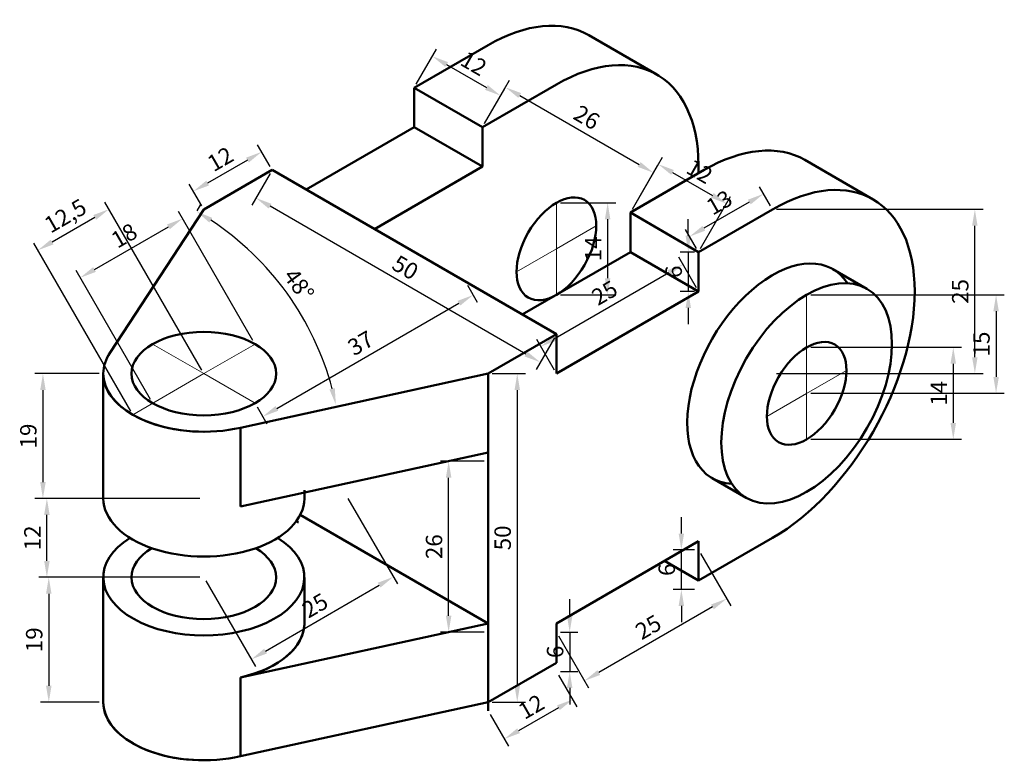
# Model space of a CAD drawing. Units: millimetres. Extents: x 225 to 375, y 60 to 173.
import ezdxf

# ---------------------------------------------------------------- set-up
doc = ezdxf.new("R2010")
doc.units = ezdxf.units.MM
doc.linetypes.add('CENTER', pattern=[50.8, 31.75, -6.35, 6.35, -6.35])
for name, color, linetype, lineweight in [('M-CNTR', 1, 'CENTER', 18), ('M-DIMS', 2, 'Continuous', 25), ('M-OUTL', 7, 'Continuous', 50)]:
    doc.layers.add(name, color=color, linetype=linetype, lineweight=lineweight)
doc.styles.get("Standard").update_dxf_attribs({"font": 'arial.ttf'})
doc.dimstyles.new('ISO-25', dxfattribs={"dimtxt": 2.5, "dimasz": 2.5, "dimexe": 1.25, "dimexo": 0.625, "dimtad": 1, "dimtxsty": 'Standard', "dimcen": 2.5, "dimadec": 0, "dimazin": 0, "dimtfac": 1, "dimtmove": 0, "dimatfit": 3, "dimfxl": 1, "dimarcsym": 0})

# ---------------------------------------------------------------- blocks, each defined once
blk = doc.blocks.new('*D1')
at = {"layer": 'Defpoints', "color": 0, "transparency": 16777216}
for p in [(252.15, 143.3), (269.41, 126), (238.15, 119.06), (296.76, 119.06), (253.46, 110.22)]:
    blk.add_point(p, dxfattribs=at)
at = {"layer": 'M-DIMS', "color": 0, "lineweight": -2, "transparency": 16777216}
blk.add_line((252.46, 143.84), (253.02, 144.8), dxfattribs=at)
blk.add_arc((230.32, 105.49), 44.14, 14.7826, 56.7544, dxfattribs=at)
at = {"layer": 'M-DIMS', "color": 0, "transparency": 16777216}
for points in [[(254.3, 142.05), (254.74, 142.76), (252.39, 143.72)], [(273.41, 116.85), (272.59, 116.66), (273.57, 114.32)]]:
    blk.add_solid(points, dxfattribs=at)
at = {"layer": 'M-DIMS', "color": 0, "transparency": 16777216, "insert": (267.68, 132.4), "char_height": 2.5, "attachment_point": 5, "rotation": 305.7685}
blk.add_mtext('48°', dxfattribs=at)
blk = doc.blocks.new('*D2')
at = {"layer": 'Defpoints', "color": 0, "transparency": 16777216}
for p in [(263.85, 150.06), (261.39, 145.79), (307.15, 125.06)]:
    blk.add_point(p, dxfattribs=at)
at = {"layer": 'M-DIMS', "color": 0, "lineweight": -2, "transparency": 16777216}
for p, q in [((263.54, 149.51), (260.76, 144.7)), ((302.52, 122.04), (263.55, 144.54)), ((306.84, 124.51), (304.06, 119.7))]:
    blk.add_line(p, q, dxfattribs=at)
at = {"layer": 'M-DIMS', "color": 0, "transparency": 16777216}
for points in [[(263.76, 144.9), (263.35, 144.17), (261.39, 145.79)], [(302.73, 122.4), (302.32, 121.67), (304.69, 120.79)]]:
    blk.add_solid(points, dxfattribs=at)
at = {"layer": 'M-DIMS', "color": 0, "transparency": 16777216, "insert": (283.99, 134.93), "char_height": 2.5, "attachment_point": 5, "rotation": 330}
blk.add_mtext('50', dxfattribs=at)
blk = doc.blocks.new('*D3')
at = {"layer": 'Defpoints', "color": 0, "transparency": 16777216}
for p in [(296.76, 119.06), (296.76, 69.06), (301.19, 69.06)]:
    blk.add_point(p, dxfattribs=at)
at = {"layer": 'M-DIMS', "color": 0, "lineweight": -2, "transparency": 16777216}
for p, q in [((297.39, 119.06), (302.44, 119.06)), ((301.19, 116.56), (301.19, 71.56)), ((297.39, 69.06), (302.44, 69.06))]:
    blk.add_line(p, q, dxfattribs=at)
at = {"layer": 'M-DIMS', "color": 0, "transparency": 16777216}
for points in [[(300.78, 116.56), (301.61, 116.56), (301.19, 119.06)], [(300.78, 71.56), (301.61, 71.56), (301.19, 69.06)]]:
    blk.add_solid(points, dxfattribs=at)
at = {"layer": 'M-DIMS', "color": 0, "transparency": 16777216, "insert": (299.29, 94.06), "char_height": 2.5, "attachment_point": 5, "rotation": 90}
blk.add_mtext('50', dxfattribs=at)
blk = doc.blocks.new('*D4')
at = {"layer": 'Defpoints', "color": 0, "transparency": 16777216}
for p in [(307.15, 79.72), (307.15, 73.72), (309.18, 73.72)]:
    blk.add_point(p, dxfattribs=at)
at = {"layer": 'M-DIMS', "color": 0, "lineweight": -2, "transparency": 16777216}
for p, q in [((309.18, 82.22), (309.18, 84.72)), ((307.78, 79.72), (310.43, 79.72)), ((309.18, 79.72), (309.18, 73.72)), ((307.78, 73.72), (310.43, 73.72)), ((309.18, 71.22), (309.18, 68.72))]:
    blk.add_line(p, q, dxfattribs=at)
at = {"layer": 'M-DIMS', "color": 0, "transparency": 16777216}
for points in [[(308.76, 82.22), (309.6, 82.22), (309.18, 79.72)], [(308.76, 71.22), (309.6, 71.22), (309.18, 73.72)]]:
    blk.add_solid(points, dxfattribs=at)
at = {"layer": 'M-DIMS', "color": 0, "transparency": 16777216, "insert": (307.28, 76.72), "char_height": 2.5, "attachment_point": 5, "rotation": 90}
blk.add_mtext('6', dxfattribs=at)
blk = doc.blocks.new('*D5')
at = {"layer": 'Defpoints', "color": 0, "transparency": 16777216}
for p in [(328.81, 92.22), (307.15, 79.72), (311.43, 72.31)]:
    blk.add_point(p, dxfattribs=at)
at = {"layer": 'M-DIMS', "color": 0, "lineweight": -2, "transparency": 16777216}
for p, q in [((329.12, 91.68), (333.71, 83.73)), ((330.92, 83.56), (313.6, 73.56)), ((307.47, 79.18), (312.06, 71.23))]:
    blk.add_line(p, q, dxfattribs=at)
at = {"layer": 'M-DIMS', "color": 0, "transparency": 16777216}
for points in [[(330.71, 83.92), (331.13, 83.2), (333.08, 84.81)], [(313.39, 73.92), (313.81, 73.2), (311.43, 72.31)]]:
    blk.add_solid(points, dxfattribs=at)
at = {"layer": 'M-DIMS', "color": 0, "transparency": 16777216, "insert": (321.31, 80.21), "char_height": 2.5, "attachment_point": 5, "rotation": 30}
blk.add_mtext('25', dxfattribs=at)
blk = doc.blocks.new('*D6')
at = {"layer": 'Defpoints', "color": 0, "transparency": 16777216}
for p in [(326.18, 92.22), (328.81, 92.22), (328.81, 86.22)]:
    blk.add_point(p, dxfattribs=at)
at = {"layer": 'M-DIMS', "color": 0, "lineweight": -2, "transparency": 16777216}
for p, q in [((326.18, 94.72), (326.18, 97.22)), ((328.18, 92.22), (324.93, 92.22)), ((326.18, 86.22), (326.18, 92.22)), ((328.18, 86.22), (324.93, 86.22)), ((326.18, 83.72), (326.18, 81.22))]:
    blk.add_line(p, q, dxfattribs=at)
at = {"layer": 'M-DIMS', "color": 0, "transparency": 16777216}
for points in [[(325.77, 94.72), (326.6, 94.72), (326.18, 92.22)], [(325.77, 83.72), (326.6, 83.72), (326.18, 86.22)]]:
    blk.add_solid(points, dxfattribs=at)
at = {"layer": 'M-DIMS', "color": 0, "transparency": 16777216, "insert": (324.28, 89.22), "char_height": 2.5, "attachment_point": 5, "rotation": 90}
blk.add_mtext('6', dxfattribs=at)
blk = doc.blocks.new('*D7')
at = {"layer": 'Defpoints', "color": 0, "transparency": 16777216}
for p in [(345.26, 123.06), (345.26, 109.06), (367.59, 109.06)]:
    blk.add_point(p, dxfattribs=at)
at = {"layer": 'M-DIMS', "color": 0, "lineweight": -2, "transparency": 16777216}
for p, q in [((345.88, 123.06), (368.84, 123.06)), ((367.59, 120.56), (367.59, 111.56)), ((345.88, 109.06), (368.84, 109.06))]:
    blk.add_line(p, q, dxfattribs=at)
at = {"layer": 'M-DIMS', "color": 0, "transparency": 16777216}
for points in [[(367.17, 120.56), (368.01, 120.56), (367.59, 123.06)], [(367.17, 111.56), (368.01, 111.56), (367.59, 109.06)]]:
    blk.add_solid(points, dxfattribs=at)
at = {"layer": 'M-DIMS', "color": 0, "transparency": 16777216, "insert": (365.71, 116.06), "char_height": 2.5, "attachment_point": 5, "rotation": 90}
blk.add_mtext('14', dxfattribs=at)
blk = doc.blocks.new('*D8')
at = {"layer": 'Defpoints', "color": 0, "transparency": 16777216}
for p in [(345.26, 131.06), (345.26, 116.06), (374.11, 116.06)]:
    blk.add_point(p, dxfattribs=at)
at = {"layer": 'M-DIMS', "color": 0, "lineweight": -2, "transparency": 16777216}
for p, q in [((345.88, 131.06), (375.36, 131.06)), ((374.11, 128.56), (374.11, 118.56)), ((345.88, 116.06), (375.36, 116.06))]:
    blk.add_line(p, q, dxfattribs=at)
at = {"layer": 'M-DIMS', "color": 0, "transparency": 16777216}
for points in [[(373.7, 128.56), (374.53, 128.56), (374.11, 131.06)], [(373.7, 118.56), (374.53, 118.56), (374.11, 116.06)]]:
    blk.add_solid(points, dxfattribs=at)
at = {"layer": 'M-DIMS', "color": 0, "transparency": 16777216, "insert": (372.21, 123.56), "char_height": 2.5, "attachment_point": 5, "rotation": 90}
blk.add_mtext('15', dxfattribs=at)
blk = doc.blocks.new('*D9')
at = {"layer": 'Defpoints', "color": 0, "transparency": 16777216}
for p in [(340.06, 144.06), (327.44, 139.92), (328.81, 137.56)]:
    blk.add_point(p, dxfattribs=at)
at = {"layer": 'M-DIMS', "color": 0, "lineweight": -2, "transparency": 16777216}
for p, q in [((339.75, 144.6), (338.07, 147.5)), ((336.53, 145.17), (329.61, 141.17)), ((328.49, 138.1), (326.82, 141))]:
    blk.add_line(p, q, dxfattribs=at)
at = {"layer": 'M-DIMS', "color": 0, "transparency": 16777216}
for points in [[(336.33, 145.53), (336.74, 144.81), (338.7, 146.42)], [(329.4, 141.53), (329.81, 140.81), (327.44, 139.92)]]:
    blk.add_solid(points, dxfattribs=at)
at = {"layer": 'M-DIMS', "color": 0, "transparency": 16777216, "insert": (332.12, 144.82), "char_height": 2.5, "attachment_point": 5, "rotation": 30}
blk.add_mtext('13', dxfattribs=at)
blk = doc.blocks.new('*D10')
at = {"layer": 'Defpoints', "color": 0, "transparency": 16777216}
for p in [(328.81, 137.56), (327.24, 131.56), (328.81, 131.56)]:
    blk.add_point(p, dxfattribs=at)
at = {"layer": 'M-DIMS', "color": 0, "lineweight": -2, "transparency": 16777216}
for p, q in [((327.24, 140.06), (327.24, 142.56)), ((328.18, 137.56), (325.99, 137.56)), ((327.24, 137.56), (327.24, 131.56)), ((328.18, 131.56), (325.99, 131.56)), ((327.24, 129.06), (327.24, 126.56))]:
    blk.add_line(p, q, dxfattribs=at)
at = {"layer": 'M-DIMS', "color": 0, "transparency": 16777216}
for points in [[(326.82, 140.06), (327.65, 140.06), (327.24, 137.56)], [(326.82, 129.06), (327.65, 129.06), (327.24, 131.56)]]:
    blk.add_solid(points, dxfattribs=at)
at = {"layer": 'M-DIMS', "color": 0, "transparency": 16777216, "insert": (325.34, 134.56), "char_height": 2.5, "attachment_point": 5, "rotation": 90}
blk.add_mtext('6', dxfattribs=at)
blk = doc.blocks.new('*D11')
at = {"layer": 'Defpoints', "color": 0, "transparency": 16777216}
for p in [(326.43, 135.68), (328.81, 131.56), (307.15, 119.06)]:
    blk.add_point(p, dxfattribs=at)
at = {"layer": 'M-DIMS', "color": 0, "lineweight": -2, "transparency": 16777216}
for p, q in [((328.49, 132.1), (325.8, 136.76)), ((306.94, 124.43), (324.26, 134.43)), ((306.84, 119.6), (304.15, 124.26))]:
    blk.add_line(p, q, dxfattribs=at)
at = {"layer": 'M-DIMS', "color": 0, "transparency": 16777216}
for points in [[(324.05, 134.79), (324.47, 134.07), (326.43, 135.68)], [(306.73, 124.79), (307.15, 124.07), (304.78, 123.18)]]:
    blk.add_solid(points, dxfattribs=at)
at = {"layer": 'M-DIMS', "color": 0, "transparency": 16777216, "insert": (314.65, 131.07), "char_height": 2.5, "attachment_point": 5, "rotation": 30}
blk.add_mtext('25', dxfattribs=at)
blk = doc.blocks.new('*D12')
at = {"layer": 'Defpoints', "color": 0, "transparency": 16777216}
for p in [(295.9, 156.56), (321.92, 149.63), (318.41, 143.56)]:
    blk.add_point(p, dxfattribs=at)
at = {"layer": 'M-DIMS', "color": 0, "lineweight": -2, "transparency": 16777216}
for p, q in [((296.21, 157.1), (300.03, 163.72)), ((301.57, 161.38), (319.76, 150.88)), ((318.73, 144.1), (322.55, 150.72))]:
    blk.add_line(p, q, dxfattribs=at)
at = {"layer": 'M-DIMS', "color": 0, "transparency": 16777216}
for points in [[(301.78, 161.75), (301.36, 161.02), (299.41, 162.63)], [(319.97, 151.25), (319.55, 150.52), (321.92, 149.63)]]:
    blk.add_solid(points, dxfattribs=at)
at = {"layer": 'M-DIMS', "color": 0, "transparency": 16777216, "insert": (311.62, 157.78), "char_height": 2.5, "attachment_point": 5, "rotation": 330}
blk.add_mtext('26', dxfattribs=at)
blk = doc.blocks.new('*D13')
at = {"layer": 'Defpoints', "color": 0, "transparency": 16777216}
for p in [(333.06, 144.93), (318.41, 143.56), (328.81, 137.56)]:
    blk.add_point(p, dxfattribs=at)
at = {"layer": 'M-DIMS', "color": 0, "lineweight": -2, "transparency": 16777216}
for p, q in [((318.73, 144.1), (323.3, 152.01)), ((324.84, 149.68), (330.9, 146.18)), ((329.12, 138.1), (333.69, 146.01))]:
    blk.add_line(p, q, dxfattribs=at)
at = {"layer": 'M-DIMS', "color": 0, "transparency": 16777216}
for points in [[(325.04, 150.04), (324.63, 149.32), (322.67, 150.93)], [(331.11, 146.54), (330.69, 145.82), (333.06, 144.93)]]:
    blk.add_solid(points, dxfattribs=at)
at = {"layer": 'M-DIMS', "color": 0, "transparency": 16777216, "insert": (328.81, 149.56), "char_height": 2.5, "attachment_point": 5, "rotation": 330}
blk.add_mtext('12', dxfattribs=at)
blk = doc.blocks.new('*D14')
at = {"layer": 'Defpoints', "color": 0, "transparency": 16777216}
for p in [(285.5, 162.56), (298.66, 161.35), (295.9, 156.56)]:
    blk.add_point(p, dxfattribs=at)
at = {"layer": 'M-DIMS', "color": 0, "lineweight": -2, "transparency": 16777216}
for p, q in [((285.82, 163.1), (288.9, 168.43)), ((290.44, 166.1), (296.5, 162.6)), ((296.21, 157.1), (299.29, 162.43))]:
    blk.add_line(p, q, dxfattribs=at)
at = {"layer": 'M-DIMS', "color": 0, "transparency": 16777216}
for points in [[(290.64, 166.46), (290.23, 165.74), (288.27, 167.35)], [(296.71, 162.96), (296.29, 162.24), (298.66, 161.35)]]:
    blk.add_solid(points, dxfattribs=at)
at = {"layer": 'M-DIMS', "color": 0, "transparency": 16777216, "insert": (294.41, 165.98), "char_height": 2.5, "attachment_point": 5, "rotation": 330}
blk.add_mtext('12', dxfattribs=at)
blk = doc.blocks.new('*D15')
at = {"layer": 'Defpoints', "color": 0, "transparency": 16777216}
for p in [(307.15, 145.06), (307.15, 131.06), (314.96, 131.06)]:
    blk.add_point(p, dxfattribs=at)
at = {"layer": 'M-DIMS', "color": 0, "lineweight": -2, "transparency": 16777216}
for p, q in [((307.78, 145.06), (316.21, 145.06)), ((314.96, 142.56), (314.96, 133.56)), ((307.78, 131.06), (316.21, 131.06))]:
    blk.add_line(p, q, dxfattribs=at)
at = {"layer": 'M-DIMS', "color": 0, "transparency": 16777216}
for points in [[(314.54, 142.56), (315.37, 142.56), (314.96, 145.06)], [(314.54, 133.56), (315.37, 133.56), (314.96, 131.06)]]:
    blk.add_solid(points, dxfattribs=at)
at = {"layer": 'M-DIMS', "color": 0, "transparency": 16777216, "insert": (313.08, 138.06), "char_height": 2.5, "attachment_point": 5, "rotation": 90}
blk.add_mtext('14', dxfattribs=at)
blk = doc.blocks.new('*D16')
at = {"layer": 'Defpoints', "color": 0, "transparency": 16777216}
for p in [(238.15, 119.06), (228.96, 100.06), (238.15, 100.06)]:
    blk.add_point(p, dxfattribs=at)
at = {"layer": 'M-DIMS', "color": 0, "lineweight": -2, "transparency": 16777216}
for p, q in [((237.53, 119.06), (227.71, 119.06)), ((228.96, 116.56), (228.96, 102.56)), ((237.53, 100.06), (227.71, 100.06))]:
    blk.add_line(p, q, dxfattribs=at)
at = {"layer": 'M-DIMS', "color": 0, "transparency": 16777216}
for points in [[(228.54, 116.56), (229.38, 116.56), (228.96, 119.06)], [(228.54, 102.56), (229.38, 102.56), (228.96, 100.06)]]:
    blk.add_solid(points, dxfattribs=at)
at = {"layer": 'M-DIMS', "color": 0, "transparency": 16777216, "insert": (227.06, 109.56), "char_height": 2.5, "attachment_point": 5, "rotation": 90}
blk.add_mtext('19', dxfattribs=at)
blk = doc.blocks.new('*D17')
at = {"layer": 'Defpoints', "color": 0, "transparency": 16777216}
for p in [(238.15, 88.06), (229.85, 69.06), (238.15, 69.06)]:
    blk.add_point(p, dxfattribs=at)
at = {"layer": 'M-DIMS', "color": 0, "lineweight": -2, "transparency": 16777216}
for p, q in [((237.53, 88.06), (228.6, 88.06)), ((229.85, 85.56), (229.85, 71.56)), ((237.53, 69.06), (228.6, 69.06))]:
    blk.add_line(p, q, dxfattribs=at)
at = {"layer": 'M-DIMS', "color": 0, "transparency": 16777216}
for points in [[(229.43, 85.56), (230.27, 85.56), (229.85, 88.06)], [(229.43, 71.56), (230.27, 71.56), (229.85, 69.06)]]:
    blk.add_solid(points, dxfattribs=at)
at = {"layer": 'M-DIMS', "color": 0, "transparency": 16777216, "insert": (227.95, 78.56), "char_height": 2.5, "attachment_point": 5, "rotation": 90}
blk.add_mtext('19', dxfattribs=at)
blk = doc.blocks.new('*D18')
at = {"layer": 'Defpoints', "color": 0, "transparency": 16777216}
for p in [(290.74, 105.72), (296.76, 105.72), (296.76, 79.72)]:
    blk.add_point(p, dxfattribs=at)
at = {"layer": 'M-DIMS', "color": 0, "lineweight": -2, "transparency": 16777216}
for p, q in [((296.14, 105.72), (289.49, 105.72)), ((290.74, 82.22), (290.74, 103.22)), ((296.14, 79.72), (289.49, 79.72))]:
    blk.add_line(p, q, dxfattribs=at)
at = {"layer": 'M-DIMS', "color": 0, "transparency": 16777216}
for points in [[(290.32, 103.22), (291.16, 103.22), (290.74, 105.72)], [(290.32, 82.22), (291.16, 82.22), (290.74, 79.72)]]:
    blk.add_solid(points, dxfattribs=at)
at = {"layer": 'M-DIMS', "color": 0, "transparency": 16777216, "insert": (288.84, 92.72), "char_height": 2.5, "attachment_point": 5, "rotation": 90}
blk.add_mtext('26', dxfattribs=at)
blk = doc.blocks.new('*D19')
at = {"layer": 'Defpoints', "color": 0, "transparency": 16777216}
for p in [(275.08, 100.6), (253.46, 88.06), (282.32, 88.13)]:
    blk.add_point(p, dxfattribs=at)
at = {"layer": 'M-DIMS', "color": 0, "lineweight": -2, "transparency": 16777216}
for p, q in [((275.4, 100.06), (282.95, 87.05)), ((253.77, 87.51), (261.33, 74.5)), ((262.86, 76.84), (280.16, 86.87))]:
    blk.add_line(p, q, dxfattribs=at)
at = {"layer": 'M-DIMS', "color": 0, "transparency": 16777216}
for points in [[(279.95, 87.23), (280.37, 86.51), (282.32, 88.13)], [(262.65, 77.2), (263.07, 76.47), (260.7, 75.58)]]:
    blk.add_solid(points, dxfattribs=at)
at = {"layer": 'M-DIMS', "color": 0, "transparency": 16777216, "insert": (270.56, 83.5), "char_height": 2.5, "attachment_point": 5, "rotation": 30.128}
blk.add_mtext('25', dxfattribs=at)
blk = doc.blocks.new('*D20')
at = {"layer": 'Defpoints', "color": 0, "transparency": 16777216}
for p in [(229.56, 100.06), (253.46, 100.06), (253.46, 88.06)]:
    blk.add_point(p, dxfattribs=at)
at = {"layer": 'M-DIMS', "color": 0, "lineweight": -2, "transparency": 16777216}
for p, q in [((252.84, 100.06), (228.31, 100.06)), ((229.56, 90.56), (229.56, 97.56)), ((252.84, 88.06), (228.31, 88.06))]:
    blk.add_line(p, q, dxfattribs=at)
at = {"layer": 'M-DIMS', "color": 0, "transparency": 16777216}
for points in [[(229.14, 97.56), (229.98, 97.56), (229.56, 100.06)], [(229.14, 90.56), (229.98, 90.56), (229.56, 88.06)]]:
    blk.add_solid(points, dxfattribs=at)
at = {"layer": 'M-DIMS', "color": 0, "transparency": 16777216, "insert": (227.68, 94.06), "char_height": 2.5, "attachment_point": 5, "rotation": 90}
blk.add_mtext('12', dxfattribs=at)
blk = doc.blocks.new('*D21')
at = {"layer": 'Defpoints', "color": 0, "transparency": 16777216}
for p in [(250.23, 142.65), (261.26, 123.56), (245.67, 114.56)]:
    blk.add_point(p, dxfattribs=at)
at = {"layer": 'M-DIMS', "color": 0, "lineweight": -2, "transparency": 16777216}
for p, q in [((260.94, 124.1), (249.61, 143.73)), ((236.81, 134.9), (248.07, 141.4)), ((245.35, 115.1), (234.02, 134.73))]:
    blk.add_line(p, q, dxfattribs=at)
at = {"layer": 'M-DIMS', "color": 0, "transparency": 16777216}
for points in [[(247.86, 141.76), (248.28, 141.04), (250.23, 142.65)], [(236.6, 135.26), (237.02, 134.54), (234.64, 133.65)]]:
    blk.add_solid(points, dxfattribs=at)
at = {"layer": 'M-DIMS', "color": 0, "transparency": 16777216, "insert": (241.49, 139.79), "char_height": 2.5, "attachment_point": 5, "rotation": 30}
blk.add_mtext('18', dxfattribs=at)
blk = doc.blocks.new('*D22')
at = {"layer": 'Defpoints', "color": 0, "transparency": 16777216}
for p in [(228.19, 137.83), (253.46, 119.06), (242.64, 112.81)]:
    blk.add_point(p, dxfattribs=at)
at = {"layer": 'M-DIMS', "color": 0, "lineweight": -2, "transparency": 16777216}
for p, q in [((253.15, 119.6), (238.39, 145.16)), ((236.85, 142.83), (230.35, 139.08)), ((242.32, 113.35), (227.56, 138.91))]:
    blk.add_line(p, q, dxfattribs=at)
at = {"layer": 'M-DIMS', "color": 0, "transparency": 16777216}
for points in [[(236.64, 143.19), (237.06, 142.47), (239.01, 144.08)], [(230.14, 139.44), (230.56, 138.72), (228.19, 137.83)]]:
    blk.add_solid(points, dxfattribs=at)
at = {"layer": 'M-DIMS', "color": 0, "transparency": 16777216, "insert": (232.54, 142.8), "char_height": 2.5, "attachment_point": 5, "rotation": 30}
blk.add_mtext('12,5', dxfattribs=at)
blk = doc.blocks.new('*D23')
at = {"layer": 'Defpoints', "color": 0, "transparency": 16777216}
for p in [(307.15, 73.72), (296.76, 67.72), (299.22, 63.46)]:
    blk.add_point(p, dxfattribs=at)
at = {"layer": 'M-DIMS', "color": 0, "lineweight": -2, "transparency": 16777216}
for p, q in [((307.47, 73.18), (310.24, 68.37)), ((307.45, 68.21), (301.39, 64.71)), ((297.08, 67.18), (299.85, 62.37))]:
    blk.add_line(p, q, dxfattribs=at)
at = {"layer": 'M-DIMS', "color": 0, "transparency": 16777216}
for points in [[(307.24, 68.57), (307.66, 67.85), (309.62, 69.46)], [(301.18, 65.07), (301.6, 64.35), (299.22, 63.46)]]:
    blk.add_solid(points, dxfattribs=at)
at = {"layer": 'M-DIMS', "color": 0, "transparency": 16777216, "insert": (303.48, 68.09), "char_height": 2.5, "attachment_point": 5, "rotation": 30}
blk.add_mtext('12', dxfattribs=at)
blk = doc.blocks.new('*D24')
at = {"layer": 'Defpoints', "color": 0, "transparency": 16777216}
for p in [(263.85, 150.06), (251.87, 146.81), (253.46, 144.06)]:
    blk.add_point(p, dxfattribs=at)
at = {"layer": 'M-DIMS', "color": 0, "lineweight": -2, "transparency": 16777216}
for p, q in [((263.54, 150.6), (261.64, 153.89)), ((260.1, 151.56), (254.04, 148.06)), ((253.15, 144.6), (251.25, 147.89))]:
    blk.add_line(p, q, dxfattribs=at)
at = {"layer": 'M-DIMS', "color": 0, "transparency": 16777216}
for points in [[(259.89, 151.92), (260.31, 151.19), (262.27, 152.81)], [(253.83, 148.42), (254.25, 147.69), (251.87, 146.81)]]:
    blk.add_solid(points, dxfattribs=at)
at = {"layer": 'M-DIMS', "color": 0, "transparency": 16777216, "insert": (256.13, 151.43), "char_height": 2.5, "attachment_point": 5, "rotation": 30}
blk.add_mtext('12', dxfattribs=at)
blk = doc.blocks.new('*D25')
at = {"layer": 'Defpoints', "color": 0, "transparency": 16777216}
for p in [(293.3, 133.06), (294.47, 131.02), (261.26, 114.56)]:
    blk.add_point(p, dxfattribs=at)
at = {"layer": 'M-DIMS', "color": 0, "lineweight": -2, "transparency": 16777216}
for p, q in [((293.61, 132.51), (295.1, 129.94)), ((264.59, 113.77), (292.31, 129.77)), ((261.57, 114.01), (263.05, 111.44))]:
    blk.add_line(p, q, dxfattribs=at)
at = {"layer": 'M-DIMS', "color": 0, "transparency": 16777216}
for points in [[(292.1, 130.13), (292.51, 129.41), (294.47, 131.02)], [(264.38, 114.13), (264.8, 113.41), (262.43, 112.52)]]:
    blk.add_solid(points, dxfattribs=at)
at = {"layer": 'M-DIMS', "color": 0, "transparency": 16777216, "insert": (277.5, 123.42), "char_height": 2.5, "attachment_point": 5, "rotation": 30}
blk.add_mtext('37', dxfattribs=at)
blk = doc.blocks.new('*D26')
at = {"layer": 'Defpoints', "color": 0, "transparency": 16777216}
for p in [(340.06, 144.06), (370.88, 144.06), (340.06, 119.06)]:
    blk.add_point(p, dxfattribs=at)
at = {"layer": 'M-DIMS', "color": 0, "lineweight": -2, "transparency": 16777216}
for p, q in [((340.69, 144.06), (372.13, 144.06)), ((370.88, 121.56), (370.88, 141.56)), ((340.69, 119.06), (372.13, 119.06))]:
    blk.add_line(p, q, dxfattribs=at)
at = {"layer": 'M-DIMS', "color": 0, "transparency": 16777216}
for points in [[(370.46, 141.56), (371.29, 141.56), (370.88, 144.06)], [(370.46, 121.56), (371.29, 121.56), (370.88, 119.06)]]:
    blk.add_solid(points, dxfattribs=at)
at = {"layer": 'M-DIMS', "color": 0, "transparency": 16777216, "insert": (368.98, 131.56), "char_height": 2.5, "attachment_point": 5, "rotation": 90}
blk.add_mtext('25', dxfattribs=at)

msp = doc.modelspace()

# ---------------------------------------------------------------- linework, layer by layer
at = {"layer": 'M-CNTR'}
for p, q in [((307.155, 138.055), (307.155, 145.055)), ((307.155, 138.055), (313.217, 141.555)), ((307.155, 138.055), (301.093, 134.555)), ((307.155, 138.055), (307.155, 131.055)), ((345.26, 116.055), (345.26, 131.055)), ((253.461, 119.055), (245.667, 123.555)), ((253.461, 119.055), (261.256, 123.555)), ((253.461, 119.055), (242.636, 112.805)), ((253.461, 119.055), (261.256, 114.555)), ((345.26, 116.055), (351.322, 119.555)), ((345.26, 116.055), (339.198, 112.555)), ((345.26, 116.055), (345.26, 109.055))]:
    msp.add_line(p, q, dxfattribs=at)
at = {"layer": 'M-OUTL'}
for p, q in [((312.072, 170.572), (322.464, 164.572)), ((296.763, 169.055), (285.504, 162.555)), ((285.504, 156.555), (285.504, 162.555)), ((285.504, 162.555), (295.897, 156.555)), ((307.155, 163.055), (295.897, 156.555)), ((285.504, 156.555), (269.05, 147.055)), ((295.897, 150.555), (285.504, 156.555)), ((295.897, 156.555), (295.897, 150.555)), ((344.981, 151.572), (355.373, 145.572)), ((263.854, 150.055), (253.461, 144.055)), ((307.155, 125.055), (263.854, 150.055)), ((279.442, 141.055), (295.897, 150.555)), ((329.672, 150.055), (318.413, 143.555)), ((239.206, 122.278), (253.461, 144.055)), ((340.064, 144.055), (328.805, 137.555)), ((318.413, 137.555), (318.413, 143.555)), ((318.413, 143.555), (328.805, 137.555)), ((318.413, 137.555), (301.959, 128.055)), ((328.805, 131.555), (318.413, 137.555)), ((328.805, 131.555), (328.805, 137.555)), ((328.805, 137.555), (328.805, 131.555)), ((354.446, 131.965), (349.249, 134.965)), ((307.155, 119.055), (328.805, 131.555)), ((307.155, 125.055), (301.959, 128.055)), ((296.763, 119.055), (307.155, 125.055)), ((307.155, 125.055), (307.155, 119.055)), ((238.152, 119.055), (238.152, 100.055)), ((296.763, 119.055), (259.043, 110.825)), ((296.763, 119.055), (296.763, 69.055)), ((296.763, 119.055), (296.763, 107.055)), ((259.043, 98.825), (259.043, 110.825)), ((296.763, 107.055), (259.043, 98.825)), ((336.074, 100.145), (330.878, 103.145)), ((268.771, 100.055), (268.771, 101.342)), ((268.154, 97.572), (296.763, 81.055)), ((267.856, 96.409), (267.527, 96.6)), ((307.155, 81.055), (328.806, 93.555)), ((328.806, 87.555), (340.064, 94.055)), ((328.806, 93.555), (328.806, 87.555)), ((328.806, 87.555), (323.609, 90.555)), ((238.152, 88.055), (238.152, 69.055)), ((268.771, 88.055), (268.771, 81.055)), ((296.763, 81.055), (259.043, 72.825)), ((307.155, 81.055), (307.155, 75.055)), ((296.763, 67.72), (296.763, 79.72)), ((296.763, 69.055), (307.155, 75.055)), ((259.043, 60.825), (259.043, 72.825)), ((296.763, 69.055), (259.043, 60.825))]:
    msp.add_line(p, q, dxfattribs=at)
for centre, major_axis, start_param, end_param in [((296.763, 144.055), (-15.309, -26.517), 3.1415927, 3.9269908), ((307.155, 138.055), (-15.309, -26.517), 2.3161838, 3.9269908), ((329.672, 125.055), (-15.309, -26.517), 3.1415927, 3.9269908), ((340.064, 119.055), (-15.309, -26.517), 0.7853982, 3.9269908), ((340.064, 119.055), (-9.186, -15.91), 2.8548361, 6.5699419), ((253.461, 119.055), (15.309, 0), 2.7684163, 3.1415927), ((253.461, 119.055), (-15.309, 0), 6.2831853, 7.8539816), ((253.461, 119.055), (15.309, 0), 3.1415927, 5.0855653), ((253.461, 100.055), (-15.309, 0), 12.5663706, 15.7079633), ((253.461, 88.055), (-15.309, 0), 5.5370274, 10.1709359), ((253.461, 88.055), (11.023, 0), 2.3711298, 3.1415927), ((253.461, 88.055), (11.023, 0), 0, 0.7704628), ((253.461, 88.055), (11.023, 0), 3.1415927, 6.2831853), ((253.461, 81.055), (15.309, 0), 5.0855653, 6.2831853), ((253.461, 81.055), (-15.309, 0), 8.437179, 9.424778), ((253.461, 69.055), (-15.309, 0), 6.2831853, 7.8539816), ((253.461, 69.055), (15.309, 0), 3.1415927, 5.0855653)]:
    msp.add_ellipse(centre, major_axis=major_axis, ratio=0.5773503, start_param=start_param, end_param=end_param, dxfattribs=at)
for centre, major_axis in [((307.155, 138.055), (-4.287, -7.425)), ((345.26, 116.055), (-9.186, -15.91)), ((253.461, 119.055), (-11.023, 0)), ((345.26, 116.055), (-4.287, -7.425))]:
    msp.add_ellipse(centre, major_axis=major_axis, ratio=0.5773503, dxfattribs=at)

# ---------------------------------------------------------------- dimensions: what is measured, and where the dimension line sits
at = {"layer": 'M-DIMS'}
for p1, p2, distance, picture, middle in [((285.504, 162.555), (295.897, 156.555), 5.534, '*D14', (294.408, 165.977)), ((295.897, 156.555), (318.413, 143.555), 7.02, '*D12', (311.616, 157.781)), ((263.854, 150.055), (253.461, 144.055), -3.175, '*D24', (256.13, 151.433)), ((318.413, 143.555), (328.805, 137.555), 8.514, '*D13', (328.806, 149.557)), ((307.155, 125.055), (263.854, 150.055), 4.93, '*D2', (283.99, 134.932)), ((340.064, 144.055), (328.805, 137.555), -2.728, '*D9', (332.12, 144.815)), ((253.461, 119.055), (242.636, 112.805), -28.897, '*D22', (232.537, 142.798)), ((245.667, 114.555), (261.256, 123.555), 22.046, '*D21', (241.488, 139.795)), ((307.155, 119.055), (328.805, 131.555), 4.759, '*D11', (314.65, 131.074)), ((261.256, 114.555), (293.298, 133.055), -2.345, '*D25', (277.499, 123.422)), ((253.461, 88.055), (275.084, 100.604), -14.424, '*D19', (270.558, 83.499)), ((328.805, 92.22), (307.155, 79.72), 8.556, '*D5', (321.307, 80.208)), ((307.155, 73.72), (296.763, 67.72), 4.923, '*D23', (303.48, 68.085))]:
    dim = msp.add_aligned_dim(p1=p1, p2=p2, distance=distance, dimstyle='ISO-25', override={"dimclrd": 0, "dimclre": 0, "dimclrt": 0}, dxfattribs=at)
    dim.commit()
    dim.dimension.update_dxf_attribs({"geometry": picture, "text_midpoint": middle})
dim = msp.add_angular_dim_2l(base=(269.405, 126.005), line1=((253.461, 110.217), (296.763, 119.055)), line2=((238.152, 119.055), (252.148, 143.297)), dimstyle='ISO-25', override={"dimclrd": 0, "dimclre": 0, "dimclrt": 0}, dxfattribs=at)
dim.commit()
dim.dimension.update_dxf_attribs({"geometry": '*D1', "text_midpoint": (267.678, 132.404)})
for base, p1, p2, override, picture, middle in [((314.956, 131.055), (307.155, 145.055), (307.155, 131.055), {"dimclrd": 0, "dimclre": 0, "dimclrt": 0}, '*D15', (313.076, 138.055)), ((370.877, 144.055), (340.064, 119.055), (340.064, 144.055), {"dimrnd": 0}, '*D26', (368.975, 131.555)), ((327.238, 131.555), (328.805, 137.555), (328.805, 131.555), {"dimclrd": 0, "dimclre": 0, "dimclrt": 0}, '*D10', (325.337, 134.555)), ((374.114, 116.055), (345.26, 131.055), (345.26, 116.055), {"dimclrd": 0, "dimclre": 0, "dimclrt": 0}, '*D8', (372.212, 123.555)), ((367.591, 109.055), (345.26, 123.055), (345.26, 109.055), {"dimclrd": 0, "dimclre": 0, "dimclrt": 0}, '*D7', (365.711, 116.055)), ((228.961, 100.055), (238.152, 119.055), (238.152, 100.055), {"dimclrd": 0, "dimclre": 0, "dimclrt": 0}, '*D16', (227.06, 109.555)), ((301.193, 69.055), (296.763, 119.055), (296.763, 69.055), {"dimclrd": 0, "dimclre": 0, "dimclrt": 0}, '*D3', (299.292, 94.055)), ((290.739, 105.72), (296.763, 79.72), (296.763, 105.72), {"dimclrd": 0, "dimclre": 0, "dimclrt": 0}, '*D18', (288.838, 92.72)), ((229.56, 100.055), (253.461, 88.055), (253.461, 100.055), {"dimclrd": 0, "dimclre": 0, "dimclrt": 0}, '*D20', (227.68, 94.055)), ((326.182, 92.22), (328.805, 86.22), (328.805, 92.22), {"dimclrd": 0, "dimclre": 0, "dimclrt": 0}, '*D6', (324.281, 89.22)), ((229.849, 69.055), (238.152, 88.055), (238.152, 69.055), {"dimclrd": 0, "dimclre": 0, "dimclrt": 0}, '*D17', (227.947, 78.555)), ((309.179, 73.72), (307.155, 79.72), (307.155, 73.72), {"dimclrd": 0, "dimclre": 0, "dimclrt": 0}, '*D4', (307.277, 76.72))]:
    dim = msp.add_linear_dim(base=base, p1=p1, p2=p2, angle=90, dimstyle='ISO-25', override=override, dxfattribs=at)
    dim.commit()
    dim.dimension.update_dxf_attribs({"geometry": picture, "text_midpoint": middle})

doc.saveas('drawing.dxf')
